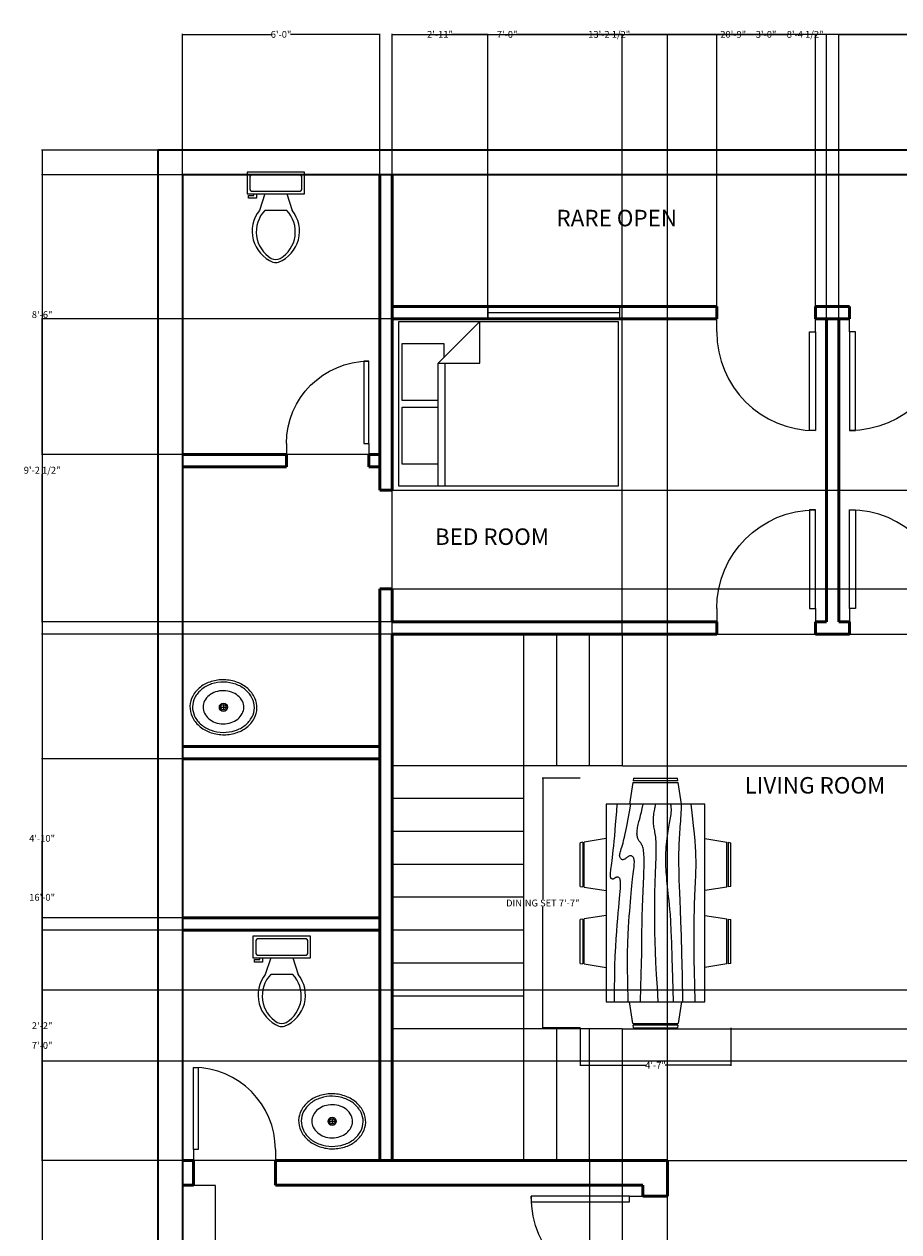
# Model space of a CAD drawing. Units: inches. Extents: x 594 to 1173, y 353 to 1285.
# Tile 4 of 6: x 595 to 914, y 844 to 1285. Entities that reach past the tile are written whole.
import ezdxf

# ---------------------------------------------------------------- set-up
doc = ezdxf.new("R2010")
doc.units = ezdxf.units.IN
doc.header["$MEASUREMENT"] = 0
for name, color, linetype, lineweight in [('A-ANNO-DIMS', 2, 'Continuous', 18), ('A-AREA-IDEN', 7, 'Continuous', 25), ('A-DOOR', 4, 'Continuous', 25), ('A-FLOR-FIXT', 9, 'Continuous', 18), ('A-FLOR-STRS', 3, 'Continuous', 25), ('A-FURN', 8, 'Continuous', 18), ('A-GLAZ', 4, 'Continuous', 25), ('A-WALL', 7, 'Continuous', 50), ('C-PROP', 7, 'Continuous', 35)]:
    doc.layers.add(name, color=color, linetype=linetype, lineweight=lineweight)
doc.styles.get("Standard").update_dxf_attribs({"font": 'arial.ttf'})
doc.dimstyles.get("Standard").update_dxf_attribs({"dimtxt": 2.5, "dimasz": 0.18, "dimexe": 0.18, "dimexo": 0.0625, "dimgap": 0.09, "dimtad": 0, "dimtih": 1, "dimtoh": 1, "dimzin": 0, "dimdsep": 46, "dimlunit": 3, "dimtxsty": 'Standard', "dimcen": 0.09, "dimadec": 0, "dimazin": 0, "dimtfac": 1, "dimtofl": 0, "dimtmove": 0, "dimatfit": 3, "dimfxl": 1, "dimtolj": 1, "dimtzin": 0, "dimarcsym": 0})

# ---------------------------------------------------------------- blocks, each defined once
blk = doc.blocks.new('*U2')
for p, q in [((0, 0), (0, -100)), ((750, 0), (750, -100))]:
    blk.add_line(p, q)
blk.add_lwpolyline([(0, 0), (0, 750), (43.75, 750), (43.75, 0)], close=True)
blk.add_arc((0, 0), 750, 0, 90)
blk = doc.blocks.new('*U4')
for p, q in [((0, 100), (0, 0)), ((900, 100), (900, 0)), ((0, 50), (900, 50))]:
    blk.add_line(p, q)
blk = doc.blocks.new('Dining Set - 36 x 72 in.')
for p, q in [((-22, 27.5), (-22.1562, 26.50042)), ((-5.8416, 26.5), (-22.1534, 26.5)), ((-22, 27.5), (-6, 27.5)), ((-5.8437, 26.49966), (-6, 27.5)), ((6, 27.5), (5.8438, 26.50042)), ((22.1584, 26.5), (5.8466, 26.5)), ((6, 27.5), (22, 27.5)), ((22.1563, 26.49966), (22, 27.5)), ((-22.2343, 26.00059), (-23.4847, 17.99762)), ((-22.2304, 26), (-5.7608, 26)), ((-4.5152, 17.99762), (-5.7655, 25.99926)), ((5.7657, 26.00059), (4.5153, 17.99762)), ((5.7696, 26), (22.2392, 26)), ((23.4848, 17.99762), (22.2345, 25.99926)), ((36, 18), (-36, 18)), ((-36, 18), (-36, -18)), ((36, -18), (36, 18)), ((-44.0006, 8.23428), (-35.9976, 9.48474)), ((44.0006, 8.23428), (35.9976, 9.48474)), ((-45.5, 8), (-44.5004, 8.15617)), ((-45.5, 8), (-45.5, -8)), ((-44.5, -8.15843), (-44.5, 8.15338)), ((-44, 8.23041), (-44, -8.23915)), ((44, 8.23041), (44, -8.23915)), ((44.5, -8.15843), (44.5, 8.15338)), ((45.5, 8), (44.5005, 8.15617)), ((45.5, 8), (45.5, -8)), ((-44.4997, -8.15631), (-45.5, -8)), ((-35.9976, -9.48476), (-43.9993, -8.2345)), ((35.9976, -9.48476), (43.9993, -8.2345)), ((44.4997, -8.15631), (45.5, -8)), ((-36, -18), (36, -18)), ((-22.2343, -26.0006), (-23.4847, -17.99762)), ((-4.5152, -17.99762), (-5.7655, -25.99928)), ((5.7657, -26.0006), (4.5153, -17.99762)), ((23.4848, -17.99762), (22.2345, -25.99928)), ((-22.2304, -26), (-5.7608, -26)), ((5.7696, -26), (22.2392, -26)), ((-22, -27.5), (-22.1562, -26.50044)), ((-5.8416, -26.5), (-22.1534, -26.5)), ((-22, -27.5), (-6, -27.5)), ((-5.8437, -26.49967), (-6, -27.5)), ((6, -27.5), (5.8438, -26.50044)), ((22.1584, -26.5), (5.8466, -26.5)), ((6, -27.5), (22, -27.5)), ((22.1563, -26.49967), (22, -27.5))]:
    blk.add_line(p, q)
for points in [[(-36, 15), (-31.1772, 14.97754), (-26.8079, 14.91406), (-22.8538, 14.81543), (-19.276, 14.6875), (-16.0362, 14.53613), (-13.0957, 14.36718), (-10.4159, 14.18652), (-7.9583, 14), (-5.6904, 13.81315), (-3.6035, 13.63021), (-1.6954, 13.45508), (0.0365, 13.29166), (1.5945, 13.14388), (2.9811, 13.01562), (4.1988, 12.9108), (5.25, 12.83333), (6.1393, 12.78613), (6.8802, 12.76823), (7.4883, 12.77767), (7.9792, 12.8125), (8.3685, 12.87077), (8.6719, 12.95052), (8.9049, 13.0498), (9.0833, 13.16666), (9.2205, 13.29899), (9.3216, 13.44401), (9.3895, 13.59879), (9.4271, 13.76041), (9.4373, 13.92594), (9.4232, 14.09245), (9.3875, 14.257), (9.3333, 14.41666), (9.2638, 14.56917), (9.1836, 14.71484), (9.0975, 14.85465), (9.0104, 14.98958), (8.9272, 15.1206), (8.8529, 15.2487), (8.7922, 15.37483), (8.75, 15.5), (8.7305, 15.62467), (8.7344, 15.74739), (8.7617, 15.86621), (8.8125, 15.97916), (8.8867, 16.08431), (8.9844, 16.17968), (9.1055, 16.26334), (9.25, 16.33333), (9.4189, 16.38802), (9.6172, 16.42708), (9.8506, 16.45052), (10.125, 16.45833), (10.4463, 16.45052), (10.8203, 16.42708), (11.2529, 16.38802), (11.75, 16.33333), (12.3184, 16.26318), (12.9694, 16.17838), (13.7151, 16.07991), (14.5677, 15.96875), (15.5395, 15.84586), (16.6426, 15.71224), (17.8893, 15.56884), (19.2917, 15.41666), (20.859, 15.25667), (22.5879, 15.08984), (24.4721, 14.91715), (26.5052, 14.73958), (28.6809, 14.5581), (30.9929, 14.3737), (33.4347, 14.18733), (36, 14)], [(-36, 10), (-28.9766, 10.14274), (-23.1725, 10.20442), (-18.4241, 10.19775), (-14.5677, 10.13541), (-11.4399, 10.03011), (-8.877, 9.89453), (-6.7154, 9.74137), (-4.7917, 9.58333), (-2.9698, 9.43082), (-1.2246, 9.28515), (0.4415, 9.14534), (2.026, 9.01041), (3.5266, 8.87939), (4.9408, 8.7513), (6.266, 8.62516), (7.5, 8.5), (8.6411, 8.37549), (9.6914, 8.2539), (10.6538, 8.13818), (11.5312, 8.03125), (12.3267, 7.93603), (13.043, 7.85547), (13.6831, 7.79248), (14.25, 7.75), (14.7471, 7.7303), (15.1797, 7.73307), (15.5537, 7.75732), (15.875, 7.80208), (16.1494, 7.86637), (16.3828, 7.94922), (16.5811, 8.04964), (16.75, 8.16666), (16.8944, 8.29915), (17.0143, 8.44531), (17.1089, 8.60319), (17.1771, 8.77083), (17.218, 8.94629), (17.2305, 9.1276), (17.2137, 9.31282), (17.1667, 9.5), (17.0895, 9.6875), (16.987, 9.875), (16.8649, 10.0625), (16.7292, 10.25), (16.5856, 10.4375), (16.4401, 10.625), (16.2985, 10.8125), (16.1667, 11), (16.05, 11.18733), (15.9518, 11.3737), (15.8752, 11.5581), (15.8229, 11.73958), (15.798, 11.91715), (15.8034, 12.08984), (15.842, 12.25667), (15.9167, 12.41666), (16.0295, 12.56836), (16.1784, 12.70833), (16.3605, 12.83268), (16.5729, 12.9375), (16.8127, 13.01888), (17.0768, 13.07291), (17.3625, 13.0957), (17.6667, 13.08333), (17.9894, 13.03312), (18.3418, 12.94726), (18.7382, 12.82918), (19.1927, 12.68229), (19.7195, 12.51001), (20.3327, 12.31575), (21.0465, 12.10294), (21.875, 11.875), (22.8357, 11.63354), (23.959, 11.37304), (25.2786, 11.08618), (26.8282, 10.76562), (28.6414, 10.40405), (30.752, 9.99414), (33.1936, 9.52856), (36, 9)], [(-36, 5.5), (-30.7157, 5.3348), (-26.069, 5.20963), (-21.9946, 5.11767), (-18.4271, 5.05208), (-15.3009, 5.00602), (-12.5508, 4.97265), (-10.1112, 4.94515), (-7.9167, 4.91666), (-5.909, 4.88167), (-4.0586, 4.83984), (-2.3429, 4.79215), (-0.7396, 4.73958), (0.7739, 4.6831), (2.22, 4.6237), (3.6213, 4.56233), (5, 4.5), (6.373, 4.43782), (7.7344, 4.3776), (9.0723, 4.32129), (10.375, 4.27083), (11.6309, 4.22819), (12.8281, 4.19531), (13.9551, 4.17415), (15, 4.16666), (15.954, 4.17448), (16.819, 4.19791), (17.6001, 4.23698), (18.3021, 4.29166), (18.9299, 4.36198), (19.4883, 4.44791), (19.9823, 4.54948), (20.4167, 4.66666), (20.7969, 4.79899), (21.1302, 4.94401), (21.4245, 5.09879), (21.6875, 5.26041), (21.9271, 5.42594), (22.1511, 5.59245), (22.3672, 5.757), (22.5834, 5.91666), (22.8065, 6.06868), (23.0404, 6.21093), (23.2879, 6.34147), (23.5521, 6.45833), (23.8358, 6.55957), (24.142, 6.64323), (24.4735, 6.70735), (24.8334, 6.75), (25.2235, 6.76969), (25.642, 6.76692), (26.0858, 6.74267), (26.5521, 6.69791), (27.0379, 6.63362), (27.5404, 6.55078), (28.0565, 6.45036), (28.5834, 6.33333), (29.1242, 6.19987), (29.7071, 6.04687), (30.3661, 5.87044), (31.1354, 5.66666), (32.0493, 5.43164), (33.142, 5.16146), (34.4475, 4.85221), (36, 4.5)], [(-36, -1), (-30.7915, -0.6591), (-26.0195, -0.38216), (-21.6519, -0.16284), (-17.6563, 0.00521), (-14.0005, 0.12833), (-10.6523, 0.21289), (-7.5796, 0.26522), (-4.75, 0.29166), (-2.134, 0.29793), (0.2878, 0.28711), (2.5317, 0.26163), (4.6146, 0.22396), (6.5529, 0.17651), (8.3633, 0.12174), (10.0623, 0.06209), (11.6667, 0), (13.1899, -0.06201), (14.6341, -0.1211), (15.9982, -0.17432), (17.2813, -0.21875), (18.4823, -0.25147), (19.6003, -0.26953), (20.6343, -0.27002), (21.5834, -0.25), (22.4481, -0.20768), (23.2357, -0.14584), (23.9549, -0.06836), (24.6146, 0.02083), (25.2235, 0.11784), (25.7904, 0.21875), (26.3241, 0.31966), (26.8334, 0.41666), (27.3265, 0.50618), (27.8099, 0.58593), (28.2894, 0.65397), (28.7709, 0.70833), (29.2601, 0.74707), (29.763, 0.76823), (30.2855, 0.76985), (30.8334, 0.75), (31.4088, 0.70784), (31.9994, 0.64713), (32.589, 0.57275), (33.1615, 0.48958), (33.7008, 0.4025), (34.1908, 0.3164), (34.6153, 0.23616), (34.9584, 0.16666), (35.2099, 0.11165), (35.3848, 0.07031), (35.504, 0.04069), (35.5886, 0.02083), (35.6594, 0.00879), (35.7377, 0.0026), (35.8442, 0.00032), (36, 0)], [(-36, -6.5), (-27.1843, -6.31267), (-20.084, -6.1263), (-14.469, -5.9419), (-10.1094, -5.76042), (-6.7752, -5.58285), (-4.2363, -5.41016), (-2.2629, -5.24333), (-0.625, -5.08334), (0.8708, -4.93099), (2.2715, -4.78646), (3.5872, -4.64974), (4.8281, -4.52084), (6.0046, -4.39974), (7.127, -4.28646), (8.2053, -4.18099), (9.25, -4.08334), (10.2705, -3.99382), (11.2734, -3.91407), (12.2647, -3.84603), (13.25, -3.79167), (14.2354, -3.75293), (15.2266, -3.73177), (16.2295, -3.73015), (17.25, -3.75), (18.2912, -3.79248), (19.3451, -3.85547), (20.4009, -3.93604), (21.4479, -4.03125), (22.4754, -4.13819), (23.4727, -4.25391), (24.4289, -4.37549), (25.3334, -4.5), (26.1785, -4.62492), (26.9694, -4.74935), (27.7145, -4.87281), (28.4219, -4.99479), (29.1, -5.11483), (29.7572, -5.23242), (30.4016, -5.34709), (31.0417, -5.45834), (31.6837, -5.56437), (32.3262, -5.65821), (32.9658, -5.73153), (33.599, -5.77604), (34.2224, -5.78345), (34.8327, -5.74545), (35.4264, -5.65373), (36, -5.5)], [(-36, -10), (-26.4022, -9.81299), (-18.4675, -9.62891), (-11.9839, -9.45069), (-6.7396, -9.28125), (-2.5226, -9.12354), (0.8789, -8.98047), (3.6769, -8.85498), (6.0833, -8.75), (8.2767, -8.66765), (10.3021, -8.60677), (12.1712, -8.56543), (13.8958, -8.54167), (15.4876, -8.53353), (16.9583, -8.53907), (18.3197, -8.55632), (19.5834, -8.58334), (20.7616, -8.61841), (21.8685, -8.66081), (22.9188, -8.71004), (23.9271, -8.76563), (24.9081, -8.82707), (25.8763, -8.89388), (26.8465, -8.96558), (27.8334, -9.04167), (28.8474, -9.12118), (29.8828, -9.20117), (30.93, -9.27824), (31.9792, -9.34896), (33.0205, -9.40991), (34.0443, -9.45768), (35.0407, -9.48885), (36, -9.5)], [(-36, -14.5), (-30.0881, -14.33513), (-25.0332, -14.21224), (-20.7312, -14.12647), (-17.0781, -14.07292), (-13.97, -14.04671), (-11.3027, -14.04297), (-8.9724, -14.05681), (-6.875, -14.08334), (-4.9224, -14.11833), (-3.0905, -14.16016), (-1.3709, -14.20785), (0.2448, -14.26042), (1.7647, -14.3169), (3.1973, -14.3763), (4.5507, -14.43767), (5.8333, -14.5), (7.0554, -14.5621), (8.235, -14.62175), (9.3922, -14.67652), (10.5469, -14.72396), (11.7192, -14.76164), (12.929, -14.78711), (14.1965, -14.79794), (15.5417, -14.79167), (16.9933, -14.76424), (18.6152, -14.70508), (20.4804, -14.60197), (22.6615, -14.44271), (25.2312, -14.21509), (28.2624, -13.9069), (31.8277, -13.50594), (36, -13)]]:
    blk.add_lwpolyline(points)
blk = doc.blocks.new('Bed - Queen')
for p, q in [((0, -80.00003), (0, 0)), ((0, 0), (59.99999, 0)), ((59.99999, 0), (59.99999, -80.00003)), ((7.99999, -1.2), (28.79998, -1.2)), ((7.99999, -14.4), (7.99999, -1.2)), ((28.79998, -1.2), (28.79998, -14.4)), ((31.19999, -1.2), (51.99999, -1.2)), ((31.19999, -14.4), (31.19999, -1.2)), ((51.99999, -1.2), (51.99999, -16.4)), ((0, -14.4), (44.8, -14.4)), ((44.8, -16.8), (0, -16.8)), ((59.99999, -29.6), (44.8, -14.4)), ((44.8, -14.4), (44.8, -29.6)), ((51.99999, -16.4), (46.79936, -16.4)), ((44.8, -29.6), (59.99999, -29.6)), ((59.99999, -80.00003), (0, -80.00003))]:
    blk.add_line(p, q)
blk = doc.blocks.new('Sink - Oval top')
for p, q in [((-1, 0), (1, 0)), ((0, 1), (0, -1))]:
    blk.add_line(p, q)
for points in [[(-12.23, 0.39, 0.117634), (-11.46, -3.36, 0.104469), (-8.88, -6.8, 0.090016), (-5.08, -9.07, 0.08192), (-0.32, -10.02, 0.08192), (4.49, -9.38, 0.090016), (8.42, -7.36, 0.104469), (11.22, -4.09, 0.117634), (12.23, -0.39, 0.117634), (11.46, 3.36, 0.104469), (8.88, 6.8, 0.090016), (5.08, 9.07, 0.08192), (0.32, 10.02, 0.08192), (-4.49, 9.38, 0.090016), (-8.42, 7.36, 0.104469), (-11.22, 4.09, 0.117634)], [(-11.29, 0.16, 0.118622), (-10.52, -3.25, 0.104678), (-8.07, -6.36, 0.089562), (-4.54, -8.37, 0.081185), (-0.13, -9.15, 0.081185), (4.3, -8.49, 0.089562), (7.89, -6.58, 0.104678), (10.42, -3.55, 0.118622), (11.29, -0.16, 0.118622), (10.52, 3.25, 0.104678), (8.07, 6.36, 0.089562), (4.54, 8.37, 0.081185), (0.13, 9.15, 0.081185), (-4.3, 8.49, 0.089562), (-7.89, 6.58, 0.104678), (-10.42, 3.55, 0.118622)], [(-7.42, 0.08, 0.118283), (-6.91, -2.17, 0.104607), (-5.29, -4.21, 0.089718), (-2.97, -5.53, 0.081436), (-0.07, -6.04, 0.081436), (2.84, -5.59, 0.089718), (5.2, -4.33, 0.104607), (6.86, -2.32, 0.118283), (7.42, -0.08, 0.118283), (6.91, 2.17, 0.104607), (5.29, 4.21, 0.089718), (2.97, 5.53, 0.081436), (0.07, 6.04, 0.081436), (-2.84, 5.59, 0.089718), (-5.2, 4.33, 0.104607), (-6.86, 2.32, 0.118283)]]:
    blk.add_lwpolyline(points, format="xyb", close=True)
for radius in [1.5, 1]:
    blk.add_circle((0, 0), radius)
blk = doc.blocks.new('Toilet - top')
for p, q in [((9.5, -6), (9.5, -2)), ((-10, -8.5), (-8, -8.5)), ((-10, -9.5), (-10, -8.5)), ((-8, -8.5), (-8, -8)), ((-7, -8), (-7, -9.5)), ((-4, -8), (-6, -14)), ((4, -8), (6, -14)), ((-7, -9.5), (-10, -9.5)), ((4, -14), (-4, -14))]:
    blk.add_line(p, q)
blk.add_lwpolyline([(10.5, -8), (10.5, 0), (-10.5, 0), (-10.5, -8)], close=True)
for points in [[(-9.5, -2), (-9.5, -6)], [(8.5, -1), (-8.5, -1)], [(-8.5, -7), (8.5, -7)]]:
    blk.add_lwpolyline(points)
for centre, radius, start, end in [((-8.62, -1.88), 0.884, 81.8699, 188.1301), ((8.62, -1.88), 0.884, 351.8699, 98.1301), ((-8.62, -6.12), 0.884, 171.8699, 278.1301), ((8.62, -6.12), 0.884, 261.8699, 8.1301), ((3.52, -21.58), 12.17, 141.4691, 247.9714), ((4.2, -21.82), 11.33, 136.3677, 238.9468), ((-3.52, -21.58), 12.17, 292.0284, 38.5307), ((-4.2, -21.82), 11.33, 301.053, 43.6321), ((0, -27.88), 4, 245.7318, 294.2682), ((0, -29), 4, 254.8605, 285.1395)]:
    blk.add_arc(centre, radius, start, end)
blk = doc.blocks.new('*D17')
at = {"layer": 'A-ANNO-DIMS', "color": 0, "lineweight": -2, "transparency": 16777216}
for p, q in [((652.4, 861.28), (664.44, 861.28)), ((664.26, 861.1), (664.26, 789.15)), ((664.26, 714.46), (664.26, 786.42)), ((652.4, 714.28), (664.44, 714.28))]:
    blk.add_line(p, q, dxfattribs=at)
at = {"layer": 'A-ANNO-DIMS', "color": 0, "transparency": 16777216}
for points in [[(664.23, 861.1), (664.29, 861.1), (664.26, 861.28)], [(664.23, 714.46), (664.29, 714.46), (664.26, 714.28)]]:
    blk.add_solid(points, dxfattribs=at)
at = {"layer": 'Defpoints', "color": 0, "transparency": 16777216}
for p in [(652.34, 861.28), (652.34, 714.28), (664.26, 714.28)]:
    blk.add_point(p, dxfattribs=at)
at = {"layer": 'A-ANNO-DIMS', "color": 0, "transparency": 16777216, "insert": (664.26, 787.78), "char_height": 2.5, "attachment_point": 5}
blk.add_mtext('\\A1;12\'-3.00"', dxfattribs=at)
blk = doc.blocks.new('WIN-FRAME-48IN')
for p, q in [((0, 0), (0, 4.5)), ((0, 4.5), (48, 4.5)), ((48, 4.5), (48, 0))]:
    blk.add_line(p, q)
blk = doc.blocks.new('*D32')
at = {"layer": 'A-ANNO-DIMS', "color": 0, "lineweight": -2, "transparency": 16777216}
for p, q in [((797.44, 1009.7), (783.67, 1009.7)), ((783.85, 1009.52), (783.85, 965.59)), ((783.85, 918.88), (783.85, 962.82)), ((797.44, 918.7), (783.67, 918.7))]:
    blk.add_line(p, q, dxfattribs=at)
at = {"layer": 'A-ANNO-DIMS', "color": 0, "transparency": 16777216}
for points in [[(783.82, 1009.52), (783.88, 1009.52), (783.85, 1009.7)], [(783.82, 918.88), (783.88, 918.88), (783.85, 918.7)]]:
    blk.add_solid(points, dxfattribs=at)
at = {"layer": 'Defpoints', "color": 0, "transparency": 16777216}
for p in [(783.85, 1009.7), (797.5, 1009.7), (797.5, 918.7)]:
    blk.add_point(p, dxfattribs=at)
at = {"layer": 'A-ANNO-DIMS', "color": 0, "transparency": 16777216, "insert": (783.85, 964.2), "char_height": 2.5, "attachment_point": 5}
blk.add_mtext('\\A1;DINING SET 7\'-7"', dxfattribs=at)
blk = doc.blocks.new('*D33')
at = {"layer": 'A-ANNO-DIMS', "color": 0, "lineweight": -2, "transparency": 16777216}
for p, q in [((797.5, 918.64), (797.5, 904.87)), ((852.5, 918.64), (852.5, 904.87)), ((797.68, 905.05), (821.54, 905.05)), ((852.32, 905.05), (828.46, 905.05))]:
    blk.add_line(p, q, dxfattribs=at)
at = {"layer": 'A-ANNO-DIMS', "color": 0, "transparency": 16777216}
for points in [[(797.68, 905.08), (797.68, 905.02), (797.5, 905.05)], [(852.32, 905.08), (852.32, 905.02), (852.5, 905.05)]]:
    blk.add_solid(points, dxfattribs=at)
at = {"layer": 'Defpoints', "color": 0, "transparency": 16777216}
for p in [(797.5, 918.7), (852.5, 918.7), (797.5, 905.05)]:
    blk.add_point(p, dxfattribs=at)
at = {"layer": 'A-ANNO-DIMS', "color": 0, "transparency": 16777216, "insert": (825, 905.05), "char_height": 2.5, "attachment_point": 5}
blk.add_mtext('\\A1;4\'-7"', dxfattribs=at)
blk = doc.blocks.new('*D47')
at = {"layer": 'A-ANNO-DIMS', "color": 0, "lineweight": -2, "transparency": 16777216}
for p, q in [((643.27, 1238.78), (600.96, 1238.78)), ((601.14, 1238.6), (601.14, 820.15)), ((601.14, 398.96), (601.14, 817.42)), ((643.27, 398.78), (600.96, 398.78))]:
    blk.add_line(p, q, dxfattribs=at)
at = {"layer": 'A-ANNO-DIMS', "color": 0, "transparency": 16777216}
for points in [[(601.11, 1238.6), (601.17, 1238.6), (601.14, 1238.78)], [(601.11, 398.96), (601.17, 398.96), (601.14, 398.78)]]:
    blk.add_solid(points, dxfattribs=at)
at = {"layer": 'Defpoints', "color": 0, "transparency": 16777216}
for p in [(601.14, 1238.78), (643.34, 1238.78), (643.34, 398.78)]:
    blk.add_point(p, dxfattribs=at)
at = {"layer": 'A-ANNO-DIMS', "color": 0, "transparency": 16777216, "insert": (601.14, 818.78), "char_height": 2.5, "attachment_point": 5}
blk.add_mtext('\\A1;70\'-0"', dxfattribs=at)
blk = doc.blocks.new('*D48')
at = {"layer": 'A-ANNO-DIMS', "color": 0, "lineweight": -2, "transparency": 16777216}
for p, q in [((652.34, 1229.85), (652.34, 1281.16)), ((652.52, 1280.98), (684.92, 1280.98)), ((724.16, 1280.98), (691.76, 1280.98)), ((724.34, 1229.85), (724.34, 1281.16))]:
    blk.add_line(p, q, dxfattribs=at)
at = {"layer": 'A-ANNO-DIMS', "color": 0, "transparency": 16777216}
for points in [[(652.52, 1281.01), (652.52, 1280.95), (652.34, 1280.98)], [(724.16, 1281.01), (724.16, 1280.95), (724.34, 1280.98)]]:
    blk.add_solid(points, dxfattribs=at)
at = {"layer": 'Defpoints', "color": 0, "transparency": 16777216}
for p in [(724.34, 1280.98), (652.34, 1229.78), (724.34, 1229.78)]:
    blk.add_point(p, dxfattribs=at)
at = {"layer": 'A-ANNO-DIMS', "color": 0, "transparency": 16777216, "insert": (688.34, 1280.98), "char_height": 2.5, "attachment_point": 5}
blk.add_mtext('\\A1;6\'-0"', dxfattribs=at)
blk = doc.blocks.new('*D49')
at = {"layer": 'A-ANNO-DIMS', "color": 0, "lineweight": -2, "transparency": 16777216}
for p, q in [((728.84, 1177.35), (728.84, 1281.16)), ((729.02, 1280.98), (800.91, 1280.98)), ((887.16, 1280.98), (815.27, 1280.98)), ((887.34, 1177.35), (887.34, 1281.16))]:
    blk.add_line(p, q, dxfattribs=at)
at = {"layer": 'A-ANNO-DIMS', "color": 0, "transparency": 16777216}
for points in [[(729.02, 1281.01), (729.02, 1280.95), (728.84, 1280.98)], [(887.16, 1281.01), (887.16, 1280.95), (887.34, 1280.98)]]:
    blk.add_solid(points, dxfattribs=at)
at = {"layer": 'Defpoints', "color": 0, "transparency": 16777216}
for p in [(887.34, 1280.98), (728.84, 1177.28), (887.34, 1177.28)]:
    blk.add_point(p, dxfattribs=at)
at = {"layer": 'A-ANNO-DIMS', "color": 0, "transparency": 16777216, "insert": (808.09, 1280.98), "char_height": 2.5, "attachment_point": 5}
blk.add_mtext('\\A1;13\'-2 1/2"', dxfattribs=at)
blk = doc.blocks.new('*D50')
at = {"layer": 'A-ANNO-DIMS', "color": 0, "lineweight": -2, "transparency": 16777216}
for p, q in [((891.84, 1177.35), (891.84, 1281.16)), ((892.02, 1280.98), (995.91, 1280.98)), ((1114.16, 1280.98), (1010.27, 1280.98)), ((1114.34, 1177.35), (1114.34, 1281.16))]:
    blk.add_line(p, q, dxfattribs=at)
at = {"layer": 'A-ANNO-DIMS', "color": 0, "transparency": 16777216}
for points in [[(892.02, 1281.01), (892.02, 1280.95), (891.84, 1280.98)], [(1114.16, 1281.01), (1114.16, 1280.95), (1114.34, 1280.98)]]:
    blk.add_solid(points, dxfattribs=at)
at = {"layer": 'Defpoints', "color": 0, "transparency": 16777216}
for p in [(1114.34, 1280.98), (891.84, 1177.28), (1114.34, 1177.28)]:
    blk.add_point(p, dxfattribs=at)
at = {"layer": 'A-ANNO-DIMS', "color": 0, "transparency": 16777216, "insert": (1003.09, 1280.98), "char_height": 2.5, "attachment_point": 5}
blk.add_mtext('\\A1;18\'-6 1/2"', dxfattribs=at)
blk = doc.blocks.new('*D51')
at = {"layer": 'A-ANNO-DIMS', "color": 0, "lineweight": -2, "transparency": 16777216}
for p, q in [((728.77, 1177.28), (600.96, 1177.28)), ((601.14, 1177.1), (601.14, 1123.42)), ((601.14, 1066.96), (601.14, 1120.65)), ((728.77, 1066.78), (600.96, 1066.78))]:
    blk.add_line(p, q, dxfattribs=at)
at = {"layer": 'A-ANNO-DIMS', "color": 0, "transparency": 16777216}
for points in [[(601.11, 1177.1), (601.17, 1177.1), (601.14, 1177.28)], [(601.11, 1066.96), (601.17, 1066.96), (601.14, 1066.78)]]:
    blk.add_solid(points, dxfattribs=at)
at = {"layer": 'Defpoints', "color": 0, "transparency": 16777216}
for p in [(601.14, 1177.28), (728.84, 1177.28), (728.84, 1066.78)]:
    blk.add_point(p, dxfattribs=at)
at = {"layer": 'A-ANNO-DIMS', "color": 0, "transparency": 16777216, "insert": (601.14, 1122.03), "char_height": 2.5, "attachment_point": 5}
blk.add_mtext('\\A1;9\'-2 1/2"', dxfattribs=at)
blk = doc.blocks.new('*D58')
at = {"layer": 'A-ANNO-DIMS', "color": 0, "lineweight": -2, "transparency": 16777216}
for p, q in [((829.34, 647.85), (829.34, 1281.16)), ((829.52, 1280.98), (873.26, 1280.98)), ((929.66, 1280.98), (885.91, 1280.98)), ((929.84, 647.85), (929.84, 1281.16))]:
    blk.add_line(p, q, dxfattribs=at)
at = {"layer": 'A-ANNO-DIMS', "color": 0, "transparency": 16777216}
for points in [[(829.52, 1281.01), (829.52, 1280.95), (829.34, 1280.98)], [(929.66, 1281.01), (929.66, 1280.95), (929.84, 1280.98)]]:
    blk.add_solid(points, dxfattribs=at)
at = {"layer": 'Defpoints', "color": 0, "transparency": 16777216}
for p in [(929.84, 1280.98), (829.34, 647.78), (929.84, 647.78)]:
    blk.add_point(p, dxfattribs=at)
at = {"layer": 'A-ANNO-DIMS', "color": 0, "transparency": 16777216, "insert": (879.59, 1280.98), "char_height": 2.5, "attachment_point": 5}
blk.add_mtext('\\A1;8\'-4 1/2"', dxfattribs=at)
blk = doc.blocks.new('*D60')
at = {"layer": 'A-ANNO-DIMS', "color": 0, "lineweight": -2, "transparency": 16777216}
for p, q in [((724.27, 954.28), (600.96, 954.28)), ((601.14, 954.1), (601.14, 913.65)), ((601.14, 870.46), (601.14, 910.92)), ((724.27, 870.28), (600.96, 870.28))]:
    blk.add_line(p, q, dxfattribs=at)
at = {"layer": 'A-ANNO-DIMS', "color": 0, "transparency": 16777216}
for points in [[(601.11, 954.1), (601.17, 954.1), (601.14, 954.28)], [(601.11, 870.46), (601.17, 870.46), (601.14, 870.28)]]:
    blk.add_solid(points, dxfattribs=at)
at = {"layer": 'Defpoints', "color": 0, "transparency": 16777216}
for p in [(601.14, 954.28), (724.34, 954.28), (724.34, 870.28)]:
    blk.add_point(p, dxfattribs=at)
at = {"layer": 'A-ANNO-DIMS', "color": 0, "transparency": 16777216, "insert": (601.14, 912.28), "char_height": 2.5, "attachment_point": 5}
blk.add_mtext('\\A1;7\'-0"', dxfattribs=at)
blk = doc.blocks.new('*D61')
at = {"layer": 'A-ANNO-DIMS', "color": 0, "lineweight": -2, "transparency": 16777216}
for p, q in [((728.84, 1062.35), (728.84, 1281.16)), ((729.02, 1280.98), (848.93, 1280.98)), ((977.66, 1280.98), (857.74, 1280.98)), ((977.84, 1062.35), (977.84, 1281.16))]:
    blk.add_line(p, q, dxfattribs=at)
at = {"layer": 'A-ANNO-DIMS', "color": 0, "transparency": 16777216}
for points in [[(729.02, 1281.01), (729.02, 1280.95), (728.84, 1280.98)], [(977.66, 1281.01), (977.66, 1280.95), (977.84, 1280.98)]]:
    blk.add_solid(points, dxfattribs=at)
at = {"layer": 'Defpoints', "color": 0, "transparency": 16777216}
for p in [(977.84, 1280.98), (728.84, 1062.28), (977.84, 1062.28)]:
    blk.add_point(p, dxfattribs=at)
at = {"layer": 'A-ANNO-DIMS', "color": 0, "transparency": 16777216, "insert": (853.34, 1280.98), "char_height": 2.5, "attachment_point": 5}
blk.add_mtext('\\A1;20\'-9"', dxfattribs=at)
blk = doc.blocks.new('*D64')
at = {"layer": 'A-ANNO-DIMS', "color": 0, "lineweight": -2, "transparency": 16777216}
for p, q in [((728.84, 1181.85), (728.84, 1281.16)), ((729.02, 1280.98), (741.93, 1280.98)), ((763.66, 1280.98), (750.74, 1280.98)), ((763.84, 1181.85), (763.84, 1281.16))]:
    blk.add_line(p, q, dxfattribs=at)
at = {"layer": 'A-ANNO-DIMS', "color": 0, "transparency": 16777216}
for points in [[(729.02, 1281.01), (729.02, 1280.95), (728.84, 1280.98)], [(763.66, 1281.01), (763.66, 1280.95), (763.84, 1280.98)]]:
    blk.add_solid(points, dxfattribs=at)
at = {"layer": 'Defpoints', "color": 0, "transparency": 16777216}
for p in [(763.84, 1280.98), (728.84, 1181.78), (763.84, 1181.78)]:
    blk.add_point(p, dxfattribs=at)
at = {"layer": 'A-ANNO-DIMS', "color": 0, "transparency": 16777216, "insert": (746.34, 1280.98), "char_height": 2.5, "attachment_point": 5}
blk.add_mtext('\\A1;2\'-11"', dxfattribs=at)
blk = doc.blocks.new('*D68')
at = {"layer": 'A-ANNO-DIMS', "color": 0, "lineweight": -2, "transparency": 16777216}
for p, q in [((847.34, 1181.85), (847.34, 1281.16)), ((847.52, 1280.98), (861.92, 1280.98)), ((883.16, 1280.98), (868.75, 1280.98)), ((883.34, 1181.85), (883.34, 1281.16))]:
    blk.add_line(p, q, dxfattribs=at)
at = {"layer": 'A-ANNO-DIMS', "color": 0, "transparency": 16777216}
for points in [[(847.52, 1281.01), (847.52, 1280.95), (847.34, 1280.98)], [(883.16, 1281.01), (883.16, 1280.95), (883.34, 1280.98)]]:
    blk.add_solid(points, dxfattribs=at)
at = {"layer": 'Defpoints', "color": 0, "transparency": 16777216}
for p in [(883.34, 1280.98), (847.34, 1181.78), (883.34, 1181.78)]:
    blk.add_point(p, dxfattribs=at)
at = {"layer": 'A-ANNO-DIMS', "color": 0, "transparency": 16777216, "insert": (865.34, 1280.98), "char_height": 2.5, "attachment_point": 5}
blk.add_mtext('\\A1;3\'-0"', dxfattribs=at)
blk = doc.blocks.new('*D70')
at = {"layer": 'A-ANNO-DIMS', "color": 0, "lineweight": -2, "transparency": 16777216}
for p, q in [((728.84, 1062.35), (728.84, 1281.16)), ((729.02, 1280.98), (767.43, 1280.98)), ((812.66, 1280.98), (774.24, 1280.98)), ((812.84, 1062.35), (812.84, 1281.16))]:
    blk.add_line(p, q, dxfattribs=at)
at = {"layer": 'A-ANNO-DIMS', "color": 0, "transparency": 16777216}
for points in [[(729.02, 1281.01), (729.02, 1280.95), (728.84, 1280.98)], [(812.66, 1281.01), (812.66, 1280.95), (812.84, 1280.98)]]:
    blk.add_solid(points, dxfattribs=at)
at = {"layer": 'Defpoints', "color": 0, "transparency": 16777216}
for p in [(812.84, 1280.98), (728.84, 1062.28), (812.84, 1062.28)]:
    blk.add_point(p, dxfattribs=at)
at = {"layer": 'A-ANNO-DIMS', "color": 0, "transparency": 16777216, "insert": (770.84, 1280.98), "char_height": 2.5, "attachment_point": 5}
blk.add_mtext('\\A1;7\'-0"', dxfattribs=at)
blk = doc.blocks.new('*D71')
at = {"layer": 'A-ANNO-DIMS', "color": 0, "lineweight": -2, "transparency": 16777216}
for p, q in [((812.9, 918.28), (1165.72, 918.28)), ((1165.54, 918.1), (1165.54, 895.65)), ((1165.54, 870.46), (1165.54, 892.92)), ((812.9, 870.28), (1165.72, 870.28))]:
    blk.add_line(p, q, dxfattribs=at)
at = {"layer": 'A-ANNO-DIMS', "color": 0, "transparency": 16777216}
for points in [[(1165.51, 918.1), (1165.57, 918.1), (1165.54, 918.28)], [(1165.51, 870.46), (1165.57, 870.46), (1165.54, 870.28)]]:
    blk.add_solid(points, dxfattribs=at)
at = {"layer": 'Defpoints', "color": 0, "transparency": 16777216}
for p in [(812.84, 918.28), (1165.54, 918.28), (812.84, 870.28)]:
    blk.add_point(p, dxfattribs=at)
at = {"layer": 'A-ANNO-DIMS', "color": 0, "transparency": 16777216, "insert": (1165.54, 894.28), "char_height": 2.5, "attachment_point": 5}
blk.add_mtext('\\A1;4\'-0"', dxfattribs=at)
blk = doc.blocks.new('*D72')
at = {"layer": 'A-ANNO-DIMS', "color": 0, "lineweight": -2, "transparency": 16777216}
for p, q in [((728.77, 1062.28), (600.96, 1062.28)), ((601.14, 1062.1), (601.14, 967.65)), ((601.14, 870.46), (601.14, 964.92)), ((728.77, 870.28), (600.96, 870.28))]:
    blk.add_line(p, q, dxfattribs=at)
at = {"layer": 'A-ANNO-DIMS', "color": 0, "transparency": 16777216}
for points in [[(601.11, 1062.1), (601.17, 1062.1), (601.14, 1062.28)], [(601.11, 870.46), (601.17, 870.46), (601.14, 870.28)]]:
    blk.add_solid(points, dxfattribs=at)
at = {"layer": 'Defpoints', "color": 0, "transparency": 16777216}
for p in [(601.14, 1062.28), (728.84, 1062.28), (728.84, 870.28)]:
    blk.add_point(p, dxfattribs=at)
at = {"layer": 'A-ANNO-DIMS', "color": 0, "transparency": 16777216, "insert": (601.14, 966.28), "char_height": 2.5, "attachment_point": 5}
blk.add_mtext('\\A1;16\'-0"', dxfattribs=at)
blk = doc.blocks.new('*D73')
at = {"layer": 'A-ANNO-DIMS', "color": 0, "lineweight": -2, "transparency": 16777216}
for p, q in [((800.84, 870.22), (800.84, 356.4)), ((812.84, 870.22), (812.84, 356.4)), ((801.02, 356.58), (803.54, 356.58)), ((812.66, 356.58), (810.13, 356.58))]:
    blk.add_line(p, q, dxfattribs=at)
at = {"layer": 'A-ANNO-DIMS', "color": 0, "transparency": 16777216}
for points in [[(801.02, 356.61), (801.02, 356.55), (800.84, 356.58)], [(812.66, 356.61), (812.66, 356.55), (812.84, 356.58)]]:
    blk.add_solid(points, dxfattribs=at)
at = {"layer": 'Defpoints', "color": 0, "transparency": 16777216}
for p in [(800.84, 870.28), (812.84, 870.28), (812.84, 356.58)]:
    blk.add_point(p, dxfattribs=at)
at = {"layer": 'A-ANNO-DIMS', "color": 0, "transparency": 16777216, "insert": (806.84, 356.58), "char_height": 2.5, "attachment_point": 5}
blk.add_mtext('\\A1;1\'-0"', dxfattribs=at)
blk = doc.blocks.new('*D74')
at = {"layer": 'A-ANNO-DIMS', "color": 0, "lineweight": -2, "transparency": 16777216}
for p, q in [((812.9, 1062.28), (1165.72, 1062.28)), ((1165.54, 1062.1), (1165.54, 1039.65)), ((1165.54, 1014.46), (1165.54, 1036.92)), ((812.9, 1014.28), (1165.72, 1014.28))]:
    blk.add_line(p, q, dxfattribs=at)
at = {"layer": 'A-ANNO-DIMS', "color": 0, "transparency": 16777216}
for points in [[(1165.51, 1062.1), (1165.57, 1062.1), (1165.54, 1062.28)], [(1165.51, 1014.46), (1165.57, 1014.46), (1165.54, 1014.28)]]:
    blk.add_solid(points, dxfattribs=at)
at = {"layer": 'Defpoints', "color": 0, "transparency": 16777216}
for p in [(812.84, 1062.28), (1165.54, 1062.28), (812.84, 1014.28)]:
    blk.add_point(p, dxfattribs=at)
at = {"layer": 'A-ANNO-DIMS', "color": 0, "transparency": 16777216, "insert": (1165.54, 1038.28), "char_height": 2.5, "attachment_point": 5}
blk.add_mtext('\\A1;4\'-0"', dxfattribs=at)
blk = doc.blocks.new('*D75')
at = {"layer": 'A-ANNO-DIMS', "color": 0, "lineweight": -2, "transparency": 16777216}
for p, q in [((724.27, 1229.78), (600.96, 1229.78)), ((601.14, 1229.6), (601.14, 1180.15)), ((601.14, 1127.96), (601.14, 1177.42)), ((720.27, 1127.78), (600.96, 1127.78))]:
    blk.add_line(p, q, dxfattribs=at)
at = {"layer": 'A-ANNO-DIMS', "color": 0, "transparency": 16777216}
for points in [[(601.11, 1229.6), (601.17, 1229.6), (601.14, 1229.78)], [(601.11, 1127.96), (601.17, 1127.96), (601.14, 1127.78)]]:
    blk.add_solid(points, dxfattribs=at)
at = {"layer": 'Defpoints', "color": 0, "transparency": 16777216}
for p in [(601.14, 1229.78), (724.34, 1229.78), (720.34, 1127.78)]:
    blk.add_point(p, dxfattribs=at)
at = {"layer": 'A-ANNO-DIMS', "color": 0, "transparency": 16777216, "insert": (601.14, 1178.78), "char_height": 2.5, "attachment_point": 5}
blk.add_mtext('\\A1;8\'-6"', dxfattribs=at)
blk = doc.blocks.new('*D76')
at = {"layer": 'A-ANNO-DIMS', "color": 0, "lineweight": -2, "transparency": 16777216}
for p, q in [((724.27, 1016.78), (600.96, 1016.78)), ((601.14, 1016.6), (601.14, 989.15)), ((601.14, 958.96), (601.14, 986.42)), ((724.27, 958.78), (600.96, 958.78))]:
    blk.add_line(p, q, dxfattribs=at)
at = {"layer": 'A-ANNO-DIMS', "color": 0, "transparency": 16777216}
for points in [[(601.11, 1016.6), (601.17, 1016.6), (601.14, 1016.78)], [(601.11, 958.96), (601.17, 958.96), (601.14, 958.78)]]:
    blk.add_solid(points, dxfattribs=at)
at = {"layer": 'Defpoints', "color": 0, "transparency": 16777216}
for p in [(601.14, 1016.78), (724.34, 1016.78), (724.34, 958.78)]:
    blk.add_point(p, dxfattribs=at)
at = {"layer": 'A-ANNO-DIMS', "color": 0, "transparency": 16777216, "insert": (601.14, 987.78), "char_height": 2.5, "attachment_point": 5}
blk.add_mtext('\\A1;4\'-10"', dxfattribs=at)
blk = doc.blocks.new('*D79')
at = {"layer": 'A-ANNO-DIMS', "color": 0, "lineweight": -2, "transparency": 16777216}
for p, q in [((1099.99, 932.38), (600.96, 932.38)), ((601.14, 932.2), (601.14, 920.81)), ((601.14, 906.73), (601.14, 918.12)), ((1099.99, 906.55), (600.96, 906.55))]:
    blk.add_line(p, q, dxfattribs=at)
at = {"layer": 'A-ANNO-DIMS', "color": 0, "transparency": 16777216}
for points in [[(601.11, 932.2), (601.17, 932.2), (601.14, 932.38)], [(601.11, 906.73), (601.17, 906.73), (601.14, 906.55)]]:
    blk.add_solid(points, dxfattribs=at)
at = {"layer": 'Defpoints', "color": 0, "transparency": 16777216}
for p in [(601.14, 932.38), (1100.05, 932.38), (1100.05, 906.55)]:
    blk.add_point(p, dxfattribs=at)
at = {"layer": 'A-ANNO-DIMS', "color": 0, "transparency": 16777216, "insert": (601.14, 919.47), "char_height": 2.5, "attachment_point": 5}
blk.add_mtext('\\A1;2\'-2"', dxfattribs=at)
blk = doc.blocks.new('*D82')
at = {"layer": 'A-ANNO-DIMS', "color": 0, "lineweight": -2, "transparency": 16777216}
for p, q in [((724.4, 1114.78), (1165.72, 1114.78)), ((1165.54, 1114.6), (1165.54, 1098.15)), ((1165.54, 1078.96), (1165.54, 1095.42)), ((724.4, 1078.78), (1165.72, 1078.78))]:
    blk.add_line(p, q, dxfattribs=at)
at = {"layer": 'A-ANNO-DIMS', "color": 0, "transparency": 16777216}
for points in [[(1165.51, 1114.6), (1165.57, 1114.6), (1165.54, 1114.78)], [(1165.51, 1078.96), (1165.57, 1078.96), (1165.54, 1078.78)]]:
    blk.add_solid(points, dxfattribs=at)
at = {"layer": 'Defpoints', "color": 0, "transparency": 16777216}
for p in [(724.34, 1114.78), (1165.54, 1114.78), (724.34, 1078.78)]:
    blk.add_point(p, dxfattribs=at)
at = {"layer": 'A-ANNO-DIMS', "color": 0, "transparency": 16777216, "insert": (1165.54, 1096.78), "char_height": 2.5, "attachment_point": 5}
blk.add_mtext('\\A1;3\'-0"', dxfattribs=at)

msp = doc.modelspace()

# ---------------------------------------------------------------- linework, layer by layer
at = {"layer": 'A-FLOR-STRS'}
for p, q in [((728.837, 1062.283), (740.837, 1062.283)), ((776.837, 1062.283), (776.837, 870.283)), ((788.837, 1062.283), (788.837, 1014.283)), ((788.837, 1062.283), (788.837, 1014.283)), ((800.837, 1062.283), (800.837, 1014.283)), ((812.837, 1062.283), (812.837, 1014.283)), ((812.837, 1014.283), (728.837, 1014.283)), ((776.837, 1002.283), (728.837, 1002.283)), ((776.837, 990.283), (728.837, 990.283)), ((776.837, 978.283), (728.837, 978.283)), ((776.837, 966.283), (728.837, 966.283)), ((776.837, 954.283), (728.837, 954.283)), ((776.837, 942.283), (728.837, 942.283)), ((776.837, 930.283), (728.837, 930.283)), ((812.837, 918.283), (728.837, 918.283)), ((788.837, 918.283), (788.837, 870.283)), ((800.837, 918.283), (800.837, 870.283)), ((812.837, 918.283), (812.837, 870.283))]:
    msp.add_line(p, q, dxfattribs=at)
at = {"layer": 'A-WALL'}
for p, q in [((724.337, 1229.783), (724.337, 1114.783)), ((728.837, 1229.783), (728.837, 1114.783)), ((847.337, 1181.783), (728.837, 1181.783)), ((847.337, 1181.783), (847.337, 1177.283)), ((883.337, 1177.283), (883.337, 1181.783)), ((895.837, 1181.783), (883.337, 1181.783)), ((895.837, 1177.283), (895.837, 1181.783)), ((847.337, 1177.283), (728.837, 1177.283)), ((895.837, 1177.283), (883.337, 1177.283)), ((887.337, 1066.783), (887.337, 1177.283)), ((891.837, 1066.783), (891.837, 1177.283)), ((690.337, 1127.783), (652.337, 1127.783)), ((690.337, 1123.283), (690.337, 1127.783)), ((724.337, 1127.783), (720.337, 1127.783)), ((720.337, 1127.783), (720.337, 1123.283)), ((690.337, 1123.283), (652.337, 1123.283)), ((724.337, 1123.283), (720.337, 1123.283)), ((724.337, 1114.783), (728.837, 1114.783)), ((728.837, 1078.783), (724.337, 1078.783)), ((724.337, 1078.783), (724.337, 1021.283)), ((728.837, 1078.783), (728.837, 1066.783)), ((728.837, 1066.783), (847.337, 1066.783)), ((847.337, 1062.283), (847.337, 1066.783)), ((883.337, 1066.783), (883.337, 1062.283)), ((883.337, 1066.783), (887.337, 1066.783)), ((891.837, 1066.783), (895.837, 1066.783)), ((895.837, 1066.783), (895.837, 1062.283)), ((728.837, 1062.283), (847.337, 1062.283)), ((728.837, 1062.283), (728.837, 1016.783)), ((883.337, 1062.283), (895.837, 1062.283)), ((724.337, 1021.283), (652.337, 1021.283)), ((724.337, 1021.283), (724.337, 870.283)), ((728.837, 1021.283), (728.837, 870.283)), ((724.337, 1016.783), (652.337, 1016.783)), ((724.337, 958.783), (652.337, 958.783)), ((724.337, 954.283), (652.337, 954.283)), ((656.337, 870.283), (652.337, 870.283)), ((656.337, 870.283), (656.337, 861.283)), ((829.337, 870.283), (686.27, 870.283)), ((686.337, 861.283), (686.337, 870.283)), ((829.337, 870.283), (829.337, 857.283)), ((656.337, 861.283), (652.337, 861.283)), ((820.337, 861.283), (686.337, 861.283)), ((820.337, 861.283), (820.337, 857.283)), ((820.337, 857.283), (829.337, 857.283))]:
    msp.add_line(p, q, dxfattribs=at)
at = {"layer": 'C-PROP'}
for p, q in [((1123.337, 1238.783), (643.337, 1238.783)), ((643.337, 1238.783), (643.337, 398.783)), ((652.337, 1229.783), (652.337, 407.783)), ((1114.337, 1229.783), (652.337, 1229.783))]:
    msp.add_line(p, q, dxfattribs=at)

# ---------------------------------------------------------------- block references
at = {"layer": 'A-DOOR'}
for p, xscale, yscale, zscale, rotation in [((883.337, 1172.483), 0.0479999999999999, 0.0479999999999999, 0.0479999999999999, 180), ((895.837, 1172.483), -0.0479999999999999, 0.0479999999999999, 0.0479999999999999, 180), ((815.547, 857.283), -0.0478936875771171, 0.0478936875771171, 0.0478936875771171, 90)]:
    msp.add_blockref('*U2', p, dxfattribs=dict(at, xscale=xscale, yscale=yscale, zscale=zscale, rotation=rotation))
for p, xscale, yscale, zscale in [((720.337, 1131.783), -0.0400000000000001, 0.0400000000000001, 0.0400000000000001), ((883.337, 1071.583), -0.0479999999999999, 0.0479999999999999, 0.0479999999999999), ((895.837, 1071.583), 0.0479999999999999, 0.0479999999999999, 0.0479999999999999), ((656.337, 874.274), 0.0399114063142643, 0.0399114063142643, 0.0399114063142643)]:
    msp.add_blockref('*U2', p, dxfattribs=dict(at, xscale=xscale, yscale=yscale, zscale=zscale))
at = {"layer": 'A-FLOR-FIXT'}
for name, p in [('Toilet - top', (686.412, 1230.783)), ('Sink - Oval top', (667.313, 1035.594)), ('Toilet - top', (688.595, 952.163)), ('Sink - Oval top', (706.992, 884.595))]:
    msp.add_blockref(name, p, dxfattribs=at)
at = {"layer": 'A-FURN'}
for name, p, rotation in [('Bed - Queen', (731.326, 1116.228), 89.99999999999999), ('Dining Set - 36 x 72 in.', (825.002, 964.204), 89.9999999999992)]:
    msp.add_blockref(name, p, dxfattribs=dict(at, rotation=rotation))
at = {"layer": 'A-GLAZ', "xscale": 0.0533333333333332, "yscale": 0.0533333333333332, "zscale": 0.0533333333333332}
msp.add_blockref('*U4', (763.837, 1176.866), dxfattribs=at)
at = {"layer": 'A-GLAZ'}
msp.add_blockref('WIN-FRAME-48IN', (763.837, 1177.283), dxfattribs=at)

# ---------------------------------------------------------------- texts
at = {"layer": 'A-AREA-IDEN'}
for s, p in [('RARE OPEN', (788.839, 1211)), ('BED ROOM', (744.482, 1094.799)), ('LIVING ROOM', (857.512, 1004.13))]:
    msp.add_text(s, height=6, dxfattribs=at).set_placement(p)

# ---------------------------------------------------------------- dimensions: what is measured, and where the dimension line sits
at = {"layer": 'A-ANNO-DIMS'}
for base, p1, p2, picture, middle in [((724.337, 1280.983), (652.337, 1229.783), (724.337, 1229.783), '*D48', (688.337, 1280.983)), ((887.337, 1280.983), (728.837, 1177.283), (887.337, 1177.283), '*D49', (808.087, 1280.983)), ((977.837, 1280.983), (728.837, 1062.283), (977.837, 1062.283), '*D61', (853.337, 1280.983)), ((763.837, 1280.983), (728.837, 1181.783), (763.837, 1181.783), '*D64', (746.337, 1280.983)), ((812.837, 1280.983), (728.837, 1062.283), (812.837, 1062.283), '*D70', (770.837, 1280.983)), ((929.837, 1280.983), (829.337, 647.783), (929.837, 647.783), '*D58', (879.587, 1280.983)), ((883.337, 1280.983), (847.337, 1181.783), (883.337, 1181.783), '*D68', (865.337, 1280.983)), ((1114.337, 1280.983), (891.837, 1177.283), (1114.337, 1177.283), '*D50', (1003.087, 1280.983)), ((812.837, 356.583), (800.837, 870.283), (812.837, 870.283), '*D73', (806.837, 356.583))]:
    dim = msp.add_linear_dim(base=base, p1=p1, p2=p2, dimstyle='Standard', override={"dimdec": 1, "dimlfac": 1, "dimrnd": 0, "dimzin": 1, "dimdsep": 46, "dimlunit": 4, "dimfrac": 2}, dxfattribs=at)
    dim.commit()
    dim.dimension.update_dxf_attribs({"geometry": picture, "text_midpoint": middle})
for base, p1, p2, angle, override, picture, middle in [((601.137, 1238.783), (643.337, 398.783), (643.337, 1238.783), 90, {"dimdec": 1, "dimlfac": 1, "dimrnd": 0, "dimzin": 1, "dimdsep": 46, "dimlunit": 4, "dimfrac": 2}, '*D47', (601.137, 818.783)), ((601.137, 1229.783), (720.337, 1127.783), (724.337, 1229.783), 90, {"dimdec": 1, "dimlfac": 1, "dimrnd": 0, "dimzin": 1, "dimdsep": 46, "dimlunit": 4, "dimfrac": 2}, '*D75', (601.137, 1178.783)), ((601.137, 1177.283), (728.837, 1066.783), (728.837, 1177.283), 90, {"dimdec": 1, "dimlfac": 1, "dimrnd": 0, "dimzin": 1, "dimdsep": 46, "dimlunit": 4, "dimfrac": 2}, '*D51', (601.137, 1122.033)), ((1165.537, 1114.783), (724.337, 1078.783), (724.337, 1114.783), 90, {"dimdec": 1, "dimlfac": 1, "dimrnd": 0, "dimzin": 1, "dimdsep": 46, "dimlunit": 4, "dimfrac": 2}, '*D82', (1165.537, 1096.783)), ((601.137, 1062.283), (728.837, 870.283), (728.837, 1062.283), 90, {"dimdec": 1, "dimlfac": 1, "dimrnd": 0, "dimzin": 1, "dimdsep": 46, "dimlunit": 4, "dimfrac": 2}, '*D72', (601.137, 966.283)), ((1165.537, 1062.283), (812.837, 1014.283), (812.837, 1062.283), 90, {"dimdec": 1, "dimlfac": 1, "dimrnd": 0, "dimzin": 1, "dimdsep": 46, "dimlunit": 4, "dimfrac": 2}, '*D74', (1165.537, 1038.283)), ((601.137, 1016.783), (724.337, 958.783), (724.337, 1016.783), 90, {"dimdec": 1, "dimlfac": 1, "dimrnd": 0, "dimzin": 1, "dimdsep": 46, "dimlunit": 4, "dimfrac": 2}, '*D76', (601.137, 987.783)), ((601.137, 954.283), (724.337, 870.283), (724.337, 954.283), 90, {"dimdec": 1, "dimlfac": 1, "dimrnd": 0, "dimzin": 1, "dimdsep": 46, "dimlunit": 4, "dimfrac": 2}, '*D60', (601.137, 912.283)), ((601.137, 932.38), (1100.051, 906.552), (1100.051, 932.38), 90, {"dimdec": 1, "dimlfac": 1, "dimrnd": 0, "dimzin": 1, "dimdsep": 46, "dimlunit": 4, "dimfrac": 2}, '*D79', (601.137, 919.466)), ((797.502, 905.054), (852.502, 918.704), (797.502, 918.704), 180, {"dimdec": 1, "dimlfac": 1, "dimrnd": 0, "dimzin": 1, "dimdsep": 46, "dimlunit": 4, "dimfrac": 2}, '*D33', (825.002, 905.054)), ((1165.537, 918.283), (812.837, 870.283), (812.837, 918.283), 90, {"dimdec": 1, "dimlfac": 1, "dimrnd": 0, "dimzin": 1, "dimdsep": 46, "dimlunit": 4, "dimfrac": 2}, '*D71', (1165.537, 894.283)), ((664.26, 714.283), (652.337, 861.283), (652.337, 714.283), 90, {"dimclrd": 0, "dimclre": 0, "dimclrt": 0}, '*D17', (664.26, 787.783))]:
    dim = msp.add_linear_dim(base=base, p1=p1, p2=p2, angle=angle, dimstyle='Standard', override=override, dxfattribs=at)
    dim.commit()
    dim.dimension.update_dxf_attribs({"geometry": picture, "text_midpoint": middle})
dim = msp.add_linear_dim(base=(783.852, 1009.704), p1=(797.502, 918.704), p2=(797.502, 1009.704), angle=90, text='DINING SET <>', dimstyle='Standard', override={"dimdec": 1, "dimlfac": 1, "dimrnd": 0, "dimzin": 1, "dimdsep": 46, "dimlunit": 4, "dimfrac": 2}, dxfattribs=at)
dim.commit()
dim.dimension.update_dxf_attribs({"geometry": '*D32', "text_midpoint": (783.852, 964.204)})

doc.saveas('drawing.dxf')
